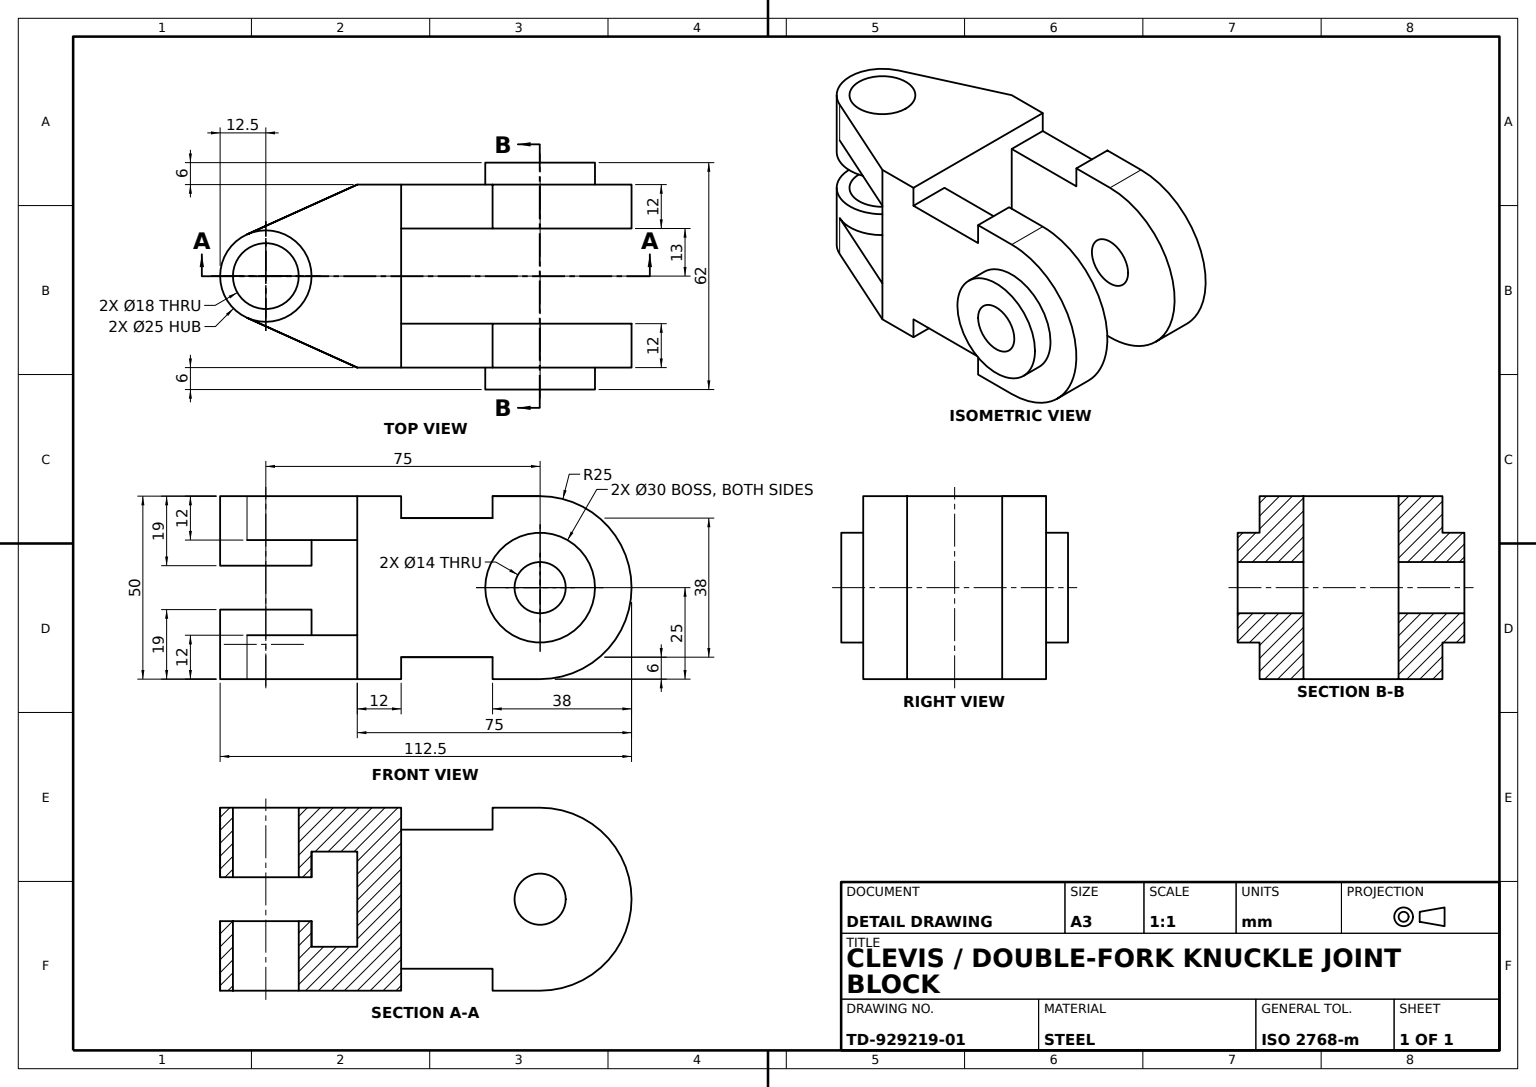
from build123d import *

# Parameters (mm, degrees)
MAIN_BODY_DEPTH              = 12
UPPER_PLATE_SKETCH_W         = 50
UPPER_PLATE_SKETCH_H         = 50
UPPER_PLATE_DEPTH            = 12
WEB_BLOCK_DEPTH              = 12
PIN_HUB_BOSS_A_SKETCH_R      = 15
PIN_HUB_BOSS_A_SKETCH_R_2    = 7
PIN_HUB_BOSS_A_30_DEPTH      = 6
PIN_START                    = -62
PIN_BORE_SKETCH_R            = 7
PIN_BORE_14_DEPTH            = 62
PIN_START_2                  = 6
PIN_HUB_BOSS_B_SKETCH_R      = 15
PIN_HUB_BOSS_B_SKETCH_R_2    = 7
PIN_HUB_BOSS_B_30_DEPTH      = 6
FORK_LUG_DEPTH               = 12
FORK_HUB_SKETCH_R            = 12.5
FORK_HUB_25_DEPTH            = 19
FORK_BORE_SKETCH_R           = 9
FORK_BORE_18_DEPTH           = 101.304536288
FORK_START                   = -12
FORK_FILLER_BLOCK_SKETCH_R   = 12.5
FORK_FILLER_BLOCK_SKETCH_R_2 = 9
FORK_FILLER_BLOCK_DEPTH      = 12
FORK_START_2                 = 7
FORK_SPACER_RING_SKETCH_R    = 12.5
FORK_SPACER_RING_SKETCH_R_2  = 9
FORK_SPACER_RING_25_DEPTH    = 7


with BuildPart() as part:
    # Main Body Side Profile Sketch → Main Body (new body)
    with BuildSketch(Plane(origin=(0, 0, 0), x_dir=(0, 0, -1), z_dir=(1, 0, 0))):
        with BuildLine():
            Line((0, 0), (0, 50))
            Line((0, 50), (12, 50))
            Line((12, 50), (12, 44))
            Line((12, 44), (37, 44))
            Line((37, 44), (37, 50))
            Line((37, 50), (50, 50))
            ThreePointArc((50, 50), (75, 25), (50, 0))
            Line((50, 0), (37, 0))
            Line((37, 0), (37, 6))
            Line((37, 6), (12, 6))
            Line((12, 6), (12, 0))
            Line((12, 0), (0, 0))
        make_face()
    extrude(amount=MAIN_BODY_DEPTH)

    # Upper Plate Sketch → Upper Plate (add)
    with BuildSketch(Plane.XY):
        with Locations((-13, 25)):
            Rectangle(UPPER_PLATE_SKETCH_W, UPPER_PLATE_SKETCH_H)
    extrude(amount=-UPPER_PLATE_DEPTH)

    # Web Block Sketch → Web Block (add)
    with BuildSketch(Plane.ZY.offset(38)):
        with BuildLine():
            Line((-12, 44), (-37, 44))
            Line((-37, 44), (-37, 50))
            Line((-37, 50), (-50, 50))
            ThreePointArc((-50, 50), (-75, 25), (-50, 0))
            Line((-50, 0), (-37, 0))
            Line((-37, 0), (-37, 6))
            Line((-37, 6), (-12, 6))
            Line((-12, 6), (-12, 44))
        make_face()
    extrude(amount=-WEB_BLOCK_DEPTH)

    # Pin Hub Boss A Sketch → Pin Hub Boss A Ø30 (add)
    with BuildSketch(Plane(origin=(12, 0, 0), x_dir=(0, 0, -1), z_dir=(1, 0, 0))):
        with Locations(Location((50, 25, 0), (0, 0, 180))):
            Circle(PIN_HUB_BOSS_A_SKETCH_R)
        with Locations((50, 25)):
            Circle(PIN_HUB_BOSS_A_SKETCH_R_2, mode=Mode.SUBTRACT)
    extrude(amount=PIN_HUB_BOSS_A_30_DEPTH)

    # Pin Bore Sketch → Pin Bore Ø14 (cut)
    with BuildSketch(Plane(origin=(12, 0, 0), x_dir=(0, 0, -1), z_dir=(1, 0, 0)).offset(PIN_START)):
        with Locations(Location((50, 25, 0), (0, 0, 180))):
            Circle(PIN_BORE_SKETCH_R)
    extrude(amount=PIN_BORE_14_DEPTH, mode=Mode.SUBTRACT)

    # Pin Hub Boss B Sketch → Pin Hub Boss B Ø30 (add)
    with BuildSketch(Plane.ZY.offset(38).offset(PIN_START_2)):
        with Locations((-50, 25)):
            Circle(PIN_HUB_BOSS_B_SKETCH_R)
        with Locations((-50, 25)):
            Circle(PIN_HUB_BOSS_B_SKETCH_R_2, mode=Mode.SUBTRACT)
    extrude(amount=-PIN_HUB_BOSS_B_30_DEPTH)

    # Fork Lug Sketch → Fork Lug (add)
    with BuildSketch(Plane(origin=(0, 50, 0), x_dir=(1, 0, 0), z_dir=(0, 1, 0))):
        with BuildLine():
            Line((-38, 0), (-24.392972847, -30.142972847))
            ThreePointArc((-24.392972847, -30.142972847), (-13, -37.5), (-1.607027153, -30.142972847))
            Line((-1.607027153, -30.142972847), (12, 0))
            Line((12, 0), (-38, 0))
        make_face()
    extrude(amount=-FORK_LUG_DEPTH)

    # Fork Hub Sketch → Fork Hub Ø25 (add)
    with BuildSketch(Plane(origin=(0, 50, 0), x_dir=(1, 0, 0), z_dir=(0, 1, 0))):
        with Locations(Location((-13, -25, 0), (0, 0, 270))):
            Circle(FORK_HUB_SKETCH_R)
    extrude(amount=-FORK_HUB_25_DEPTH)

    # Fork Bore Sketch → Fork Bore Ø18 (cut, through all)
    with BuildSketch(Plane(origin=(0, 50, 0), x_dir=(1, 0, 0), z_dir=(0, 1, 0))):
        with Locations(Location((-13, -25, 0), (0, 0, 270))):
            Circle(FORK_BORE_SKETCH_R)
    extrude(amount=-FORK_BORE_18_DEPTH, mode=Mode.SUBTRACT)

    # Fork Filler Block Sketch → Fork Filler Block (add)
    # profile 1 of 2: a face of its own
    with BuildSketch(Plane.XZ.offset(FORK_START)):
        with BuildLine():
            Line((-24.392972847, 30.142972847), (-38, 0))
            Line((-38, 0), (12, 0))
            Line((12, 0), (-1.607027153, 30.142972847))
            ThreePointArc((-1.607027153, 30.142972847), (-0.779890332, 27.630383946), (-0.5, 25))
            ThreePointArc((-0.5, 25), (-15.630383946, 12.779890332), (-24.392972847, 30.142972847))
        make_face()
    # profile 2 of 2: a face of its own
    with BuildSketch(Plane.XZ.offset(FORK_START)):
        with Locations(Location((-13, 25, 0), (0, 0, 90))):
            Circle(FORK_FILLER_BLOCK_SKETCH_R)
        with Locations(Location((-13, 25, 0), (0, 0, 90))):
            Circle(FORK_FILLER_BLOCK_SKETCH_R_2, mode=Mode.SUBTRACT)
    extrude(amount=FORK_FILLER_BLOCK_DEPTH)

    # Fork Spacer Ring Sketch → Fork Spacer Ring Ø25 (add)
    with BuildSketch(Plane(origin=(0, 12, 0), x_dir=(1, 0, 0), z_dir=(0, 1, 0)).offset(FORK_START_2)):
        with Locations(Location((-13, -25, 0), (0, 0, 270))):
            Circle(FORK_SPACER_RING_SKETCH_R)
        with Locations(Location((-13, -25, 0), (0, 0, 270))):
            Circle(FORK_SPACER_RING_SKETCH_R_2, mode=Mode.SUBTRACT)
    extrude(amount=-FORK_SPACER_RING_25_DEPTH)


solid = part.part
